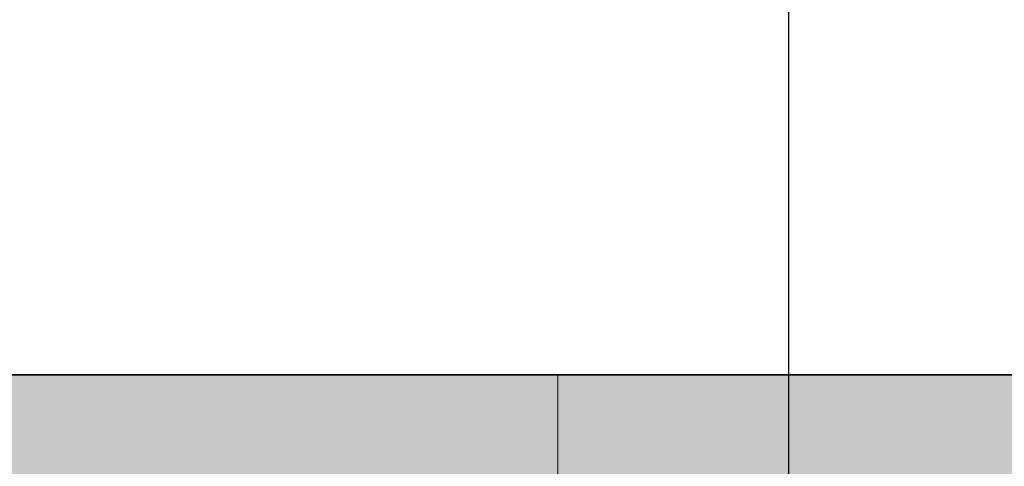
# Model space of a CAD drawing. Units: inches. Extents: x 1704 to 6393, y -157 to 1172.
# Tile 83 of 122: x 2048 to 2081, y 1030 to 1045. Entities that reach past the tile are written whole.
import ezdxf

# ---------------------------------------------------------------- set-up
doc = ezdxf.new("R2010")
doc.units = ezdxf.units.IN
doc.header["$MEASUREMENT"] = 0
for name, color, linetype, lineweight in [('A-ANNO-DIMS', 7, 'Continuous', 13), ('C-PROP', 7, 'Continuous', 35), ('L-DECK-PLNK-PATT', 250, 'Continuous', 13), ('L-HRDS', 8, 'Continuous', 18)]:
    doc.layers.add(name, color=color, linetype=linetype, lineweight=lineweight)
doc.layers.add('L-DECK-PATT', color=35, linetype='Continuous', lineweight=13, true_color=0xa6725b)
doc.layers.add('L-HRDS-PATT', color=9, linetype='Continuous', lineweight=13, true_color=0xc5c1ba)
doc.styles.get("Standard").update_dxf_attribs({"font": 'arial.ttf'})
doc.dimstyles.get("Standard").update_dxf_attribs({"dimtxt": 6, "dimasz": 2, "dimexe": 0.18, "dimexo": 0.0625, "dimgap": 0.09, "dimtad": 0, "dimtih": 1, "dimtoh": 1, "dimdec": 1, "dimzin": 0, "dimdsep": 46, "dimlunit": 3, "dimtxsty": 'Standard', "dimblk": 'ARCHTICK', "dimcen": 0.09, "dimadec": 0, "dimazin": 0, "dimtfac": 1, "dimtdec": 1, "dimtofl": 0, "dimtmove": 0, "dimatfit": 3, "dimfxl": 1, "dimtolj": 1, "dimtzin": 0, "dimarcsym": 0})

# ---------------------------------------------------------------- blocks, each defined once
blk = doc.blocks.new('_ArchTick')
at = {"color": 0, "linetype": 'ByBlock', "const_width": 0.15}
blk.add_lwpolyline([(-0.5, -0.5), (0.5, 0.5)], dxfattribs=at)
blk = doc.blocks.new('*D92')
at = {"layer": 'A-ANNO-DIMS', "color": 0, "lineweight": -2, "transparency": 16777216}
for p, q in [((2073.349, 895.275), (2073.349, 1105.287)), ((2073.349, 1105.107), (2332.661, 1105.107)), ((2605.349, 1105.107), (2346.036, 1105.107)), ((2605.349, 895.275), (2605.349, 1105.287))]:
    blk.add_line(p, q, dxfattribs=at)
at = {"layer": 'Defpoints', "color": 0, "lineweight": -3, "transparency": 16777216}
for p in [(2605.349, 1105.107), (2073.349, 895.213), (2605.349, 895.213)]:
    blk.add_point(p, dxfattribs=at)
at = {"layer": 'A-ANNO-DIMS', "color": 0, "lineweight": -2, "transparency": 16777216, "xscale": 2, "yscale": 2, "zscale": 2, "rotation": 180}
blk.add_blockref('_ArchTick', (2073.349, 1105.107), dxfattribs=at)
at = {"layer": 'A-ANNO-DIMS', "color": 0, "lineweight": -2, "transparency": 16777216, "xscale": 2, "yscale": 2, "zscale": 2}
blk.add_blockref('_ArchTick', (2605.349, 1105.107), dxfattribs=at)
at = {"layer": 'A-ANNO-DIMS', "color": 0, "transparency": 16777216, "insert": (2339.349, 1105.107), "char_height": 6, "attachment_point": 5}
blk.add_mtext('\\A1;532', dxfattribs=at)
blk = doc.blocks.new('*D94')
at = {"layer": 'A-ANNO-DIMS', "color": 0, "lineweight": -2, "transparency": 16777216}
for p, q in [((1898.349, 895.275), (1898.349, 1105.287)), ((1898.349, 1105.107), (1979.39, 1105.107)), ((2073.349, 1105.107), (1992.307, 1105.107)), ((2073.349, 895.275), (2073.349, 1105.287))]:
    blk.add_line(p, q, dxfattribs=at)
at = {"layer": 'Defpoints', "color": 0, "lineweight": -3, "transparency": 16777216}
for p in [(2073.349, 1105.107), (1898.349, 895.213), (2073.349, 895.213)]:
    blk.add_point(p, dxfattribs=at)
at = {"layer": 'A-ANNO-DIMS', "color": 0, "lineweight": -2, "transparency": 16777216, "xscale": 2, "yscale": 2, "zscale": 2, "rotation": 180}
blk.add_blockref('_ArchTick', (1898.349, 1105.107), dxfattribs=at)
at = {"layer": 'A-ANNO-DIMS', "color": 0, "lineweight": -2, "transparency": 16777216, "xscale": 2, "yscale": 2, "zscale": 2}
blk.add_blockref('_ArchTick', (2073.349, 1105.107), dxfattribs=at)
at = {"layer": 'A-ANNO-DIMS', "color": 0, "transparency": 16777216, "insert": (1985.849, 1105.107), "char_height": 6, "attachment_point": 5}
blk.add_mtext('\\A1;175', dxfattribs=at)

msp = doc.modelspace()

# ---------------------------------------------------------------- hatches: boundary and pattern name
at = {"layer": 'L-DECK-PATT', "transparency": 33554544}
h = msp.add_hatch(color=256, dxfattribs=at)
h.dxf.hatch_style = 1
h.paths.add_polyline_path([(2329.589, 1033.213), (2065.589, 1033.213), (2065.589, 895.213), (2167.349, 895.213), (2263.349, 895.213), (2263.349, 903.213), (2273.349, 903.213), (2273.349, 895.213), (2329.589, 895.213)])
h.paths.add_polyline_path([(2664.349, 1033.213), (2333.589, 1033.213), (2333.589, 895.213), (2465.349, 895.213), (2469.181, 895.213), (2470.482, 895.213), (2508.215, 895.213), (2509.516, 895.213), (2513.349, 895.213), (2533.349, 895.213), (2581.349, 895.213), (2605.349, 895.213), (2664.349, 895.213)])
h.paths.add_polyline_path([(2333.589, 1033.213), (2329.589, 1033.213), (2329.589, 895.213), (2333.589, 895.213)])
at = {"layer": 'L-DECK-PLNK-PATT'}
h = msp.add_hatch(dxfattribs=at)
h.set_pattern_fill('LINE', color=256, scale=60)
h.paths.add_polyline_path([(2329.589, 1033.213), (2065.589, 1033.213), (2065.589, 895.213), (2167.349, 895.213), (2263.349, 895.213), (2263.349, 903.213), (2273.349, 903.213), (2273.349, 895.213), (2329.589, 895.213)])
h.paths.add_polyline_path([(2664.349, 1033.213), (2333.589, 1033.213), (2333.589, 895.213), (2465.349, 895.213), (2469.181, 895.213), (2470.482, 895.213), (2508.215, 895.213), (2509.516, 895.213), (2513.349, 895.213), (2533.349, 895.213), (2581.349, 895.213), (2605.349, 895.213), (2664.349, 895.213)])
h.paths.add_polyline_path([(2333.589, 1033.213), (2329.589, 1033.213), (2329.589, 895.213), (2333.589, 895.213)])
at = {"layer": 'L-HRDS-PATT', "transparency": 33554643}
h = msp.add_hatch(color=256, dxfattribs=at)
h.dxf.hatch_style = 1
h.paths.add_polyline_path([(2065.589, 1033.213), (1898.349, 1033.213), (1898.349, 895.213), (2065.589, 895.213)])

# ---------------------------------------------------------------- linework, layer by layer
at = {"layer": 'C-PROP'}
msp.add_line((2723.349, 1033.213), (1898.349, 1033.213), dxfattribs=at)
at = {"layer": 'L-HRDS'}
msp.add_line((2065.589, 895.213), (2065.589, 1033.213), dxfattribs=at)

# ---------------------------------------------------------------- dimensions: what is measured, and where the dimension line sits
at = {"layer": 'A-ANNO-DIMS'}
for base, p1, p2, picture, middle in [((2073.349, 1105.107), (1898.349, 895.213), (2073.349, 895.213), '*D94', (1985.849, 1105.107)), ((2605.349, 1105.107), (2073.349, 895.213), (2605.349, 895.213), '*D92', (2339.349, 1105.107))]:
    dim = msp.add_linear_dim(base=base, p1=p1, p2=p2, dimstyle='Standard', override={"dimdec": 0, "dimlfac": 1, "dimrnd": 0, "dimzin": 0, "dimdsep": 46, "dimlunit": 2}, dxfattribs=at)
    dim.commit()
    dim.dimension.update_dxf_attribs({"geometry": picture, "text_midpoint": middle})

doc.saveas('drawing.dxf')
